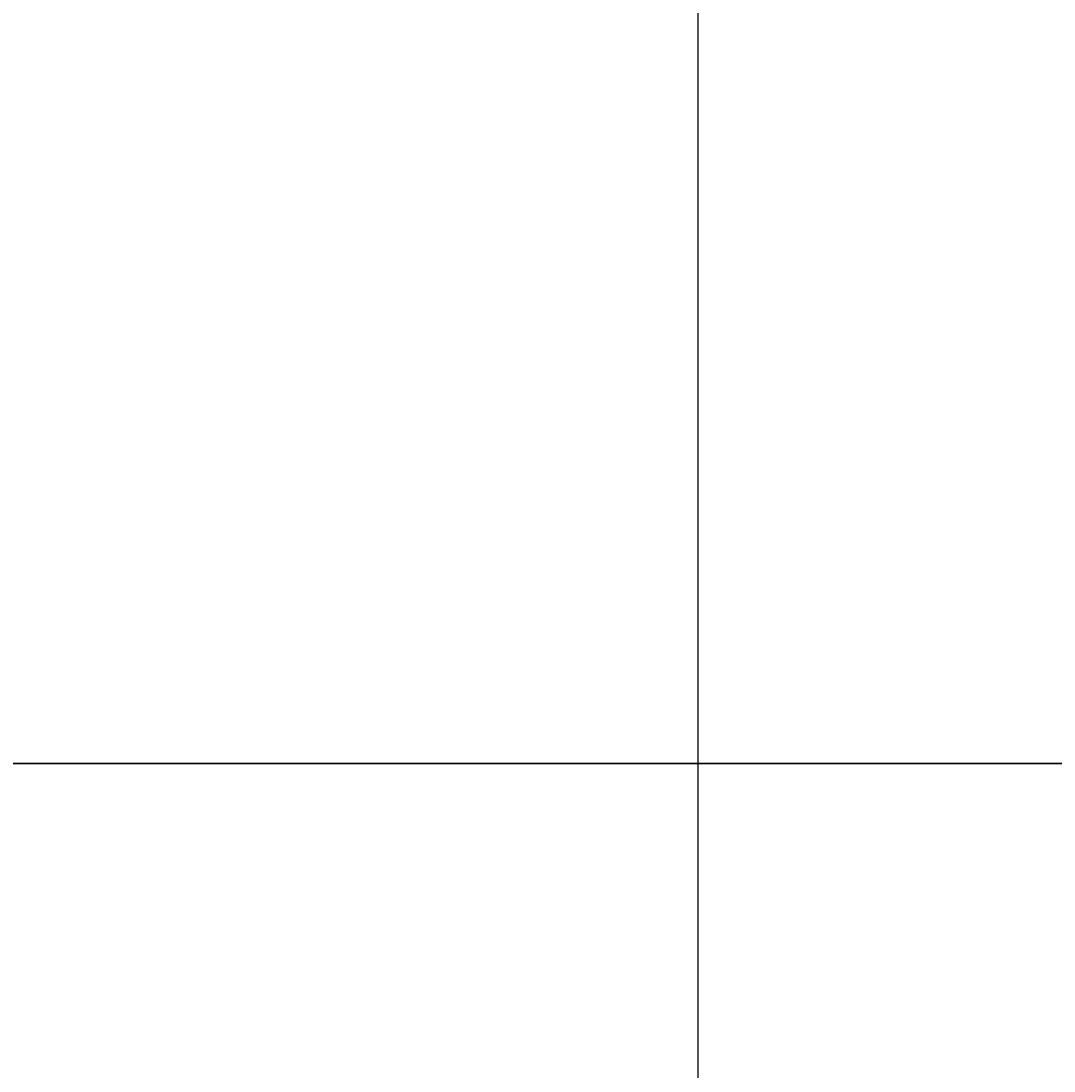
# Model space of a CAD drawing. Units: inches. Extents: x -6 to 289, y -8 to 323.
# Tile 84 of 107: x 173 to 196, y 252 to 276. Entities that reach past the tile are written whole.
import ezdxf

# ---------------------------------------------------------------- set-up
doc = ezdxf.new("R2010")
doc.units = ezdxf.units.IN
doc.header["$MEASUREMENT"] = 0
doc.layers.add('A-ANNO-DIMS', color=2, linetype='Continuous', lineweight=18)
doc.layers.add('A-ELEV', color=7, linetype='Continuous', lineweight=35)
doc.styles.get("Standard").update_dxf_attribs({"font": 'arial.ttf'})
doc.dimstyles.get("Standard").update_dxf_attribs({"dimtxt": 0.18, "dimasz": 0.18, "dimexe": 0.18, "dimexo": 0.0625, "dimgap": 0.09, "dimtad": 0, "dimtih": 1, "dimtoh": 1, "dimdec": 4, "dimzin": 0, "dimdsep": 46, "dimtxsty": 'Standard', "dimcen": 0.09, "dimadec": 0, "dimazin": 0, "dimtfac": 1, "dimtdec": 4, "dimtofl": 0, "dimtmove": 0, "dimatfit": 3, "dimfxl": 1, "dimtolj": 1, "dimtzin": 0, "dimarcsym": 0})

# ---------------------------------------------------------------- blocks, each defined once
blk = doc.blocks.new('*D12')
at = {"layer": 'A-ANNO-DIMS', "color": 0, "lineweight": -2, "transparency": 16777216}
for p, q in [((168.883, 226.717), (168.883, 322.969)), ((188.292, 226.951), (188.292, 322.969)), ((169.063, 322.789), (178.22, 322.789)), ((188.112, 322.789), (178.955, 322.789))]:
    blk.add_line(p, q, dxfattribs=at)
at = {"layer": 'A-ANNO-DIMS', "color": 0, "transparency": 16777216}
for points in [[(169.063, 322.819), (169.063, 322.759), (168.883, 322.789)], [(188.112, 322.819), (188.112, 322.759), (188.292, 322.789)]]:
    blk.add_solid(points, dxfattribs=at)
at = {"layer": 'Defpoints', "color": 0, "transparency": 16777216}
for p in [(188.292, 322.789), (188.292, 226.889), (168.883, 226.654)]:
    blk.add_point(p, dxfattribs=at)
at = {"layer": 'A-ANNO-DIMS', "color": 0, "transparency": 16777216, "insert": (178.588, 322.789), "char_height": 0.18, "attachment_point": 5}
blk.add_mtext('\\A1;19.41', dxfattribs=at)
blk = doc.blocks.new('*D13')
at = {"layer": 'A-ANNO-DIMS', "color": 0, "lineweight": -2, "transparency": 16777216}
for p, q in [((188.292, 226.951), (188.292, 322.969)), ((236.292, 226.951), (236.292, 322.969)), ((188.472, 322.789), (212.069, 322.789)), ((236.112, 322.789), (212.515, 322.789))]:
    blk.add_line(p, q, dxfattribs=at)
at = {"layer": 'A-ANNO-DIMS', "color": 0, "transparency": 16777216}
for points in [[(188.472, 322.819), (188.472, 322.759), (188.292, 322.789)], [(236.112, 322.819), (236.112, 322.759), (236.292, 322.789)]]:
    blk.add_solid(points, dxfattribs=at)
at = {"layer": 'Defpoints', "color": 0, "transparency": 16777216}
for p in [(236.292, 322.789), (188.292, 226.889), (236.292, 226.889)]:
    blk.add_point(p, dxfattribs=at)
at = {"layer": 'A-ANNO-DIMS', "color": 0, "transparency": 16777216, "insert": (212.292, 322.789), "char_height": 0.18, "attachment_point": 5}
blk.add_mtext('\\A1;48', dxfattribs=at)
blk = doc.blocks.new('*D27')
at = {"layer": 'A-ANNO-DIMS', "color": 0, "lineweight": -2, "transparency": 16777216}
for p, q in [((19.226, 307.289), (288.653, 307.289)), ((288.473, 307.109), (288.473, 277.471)), ((288.473, 247.469), (288.473, 277.107)), ((247.226, 247.289), (288.653, 247.289))]:
    blk.add_line(p, q, dxfattribs=at)
at = {"layer": 'A-ANNO-DIMS', "color": 0, "transparency": 16777216}
for points in [[(288.443, 307.109), (288.503, 307.109), (288.473, 307.289)], [(288.443, 247.469), (288.503, 247.469), (288.473, 247.289)]]:
    blk.add_solid(points, dxfattribs=at)
at = {"layer": 'Defpoints', "color": 0, "transparency": 16777216}
for p in [(19.164, 307.289), (288.473, 307.289), (247.164, 247.289)]:
    blk.add_point(p, dxfattribs=at)
at = {"layer": 'A-ANNO-DIMS', "color": 0, "transparency": 16777216, "insert": (288.473, 277.289), "char_height": 0.18, "attachment_point": 5}
blk.add_mtext('\\A1;60', dxfattribs=at)
blk = doc.blocks.new('*D79')
at = {"layer": 'A-ANNO-DIMS', "color": 0, "lineweight": -2, "transparency": 16777216}
for p, q in [((171.296, 118.033), (171.296, 322.969)), ((188.292, 116.842), (188.292, 322.969)), ((171.476, 322.789), (179.339, 322.789)), ((188.112, 322.789), (180.249, 322.789))]:
    blk.add_line(p, q, dxfattribs=at)
at = {"layer": 'A-ANNO-DIMS', "color": 0, "transparency": 16777216}
for points in [[(171.476, 322.819), (171.476, 322.759), (171.296, 322.789)], [(188.112, 322.819), (188.112, 322.759), (188.292, 322.789)]]:
    blk.add_solid(points, dxfattribs=at)
at = {"layer": 'Defpoints', "color": 0, "transparency": 16777216}
for p in [(188.292, 322.789), (171.296, 117.971), (188.292, 116.779)]:
    blk.add_point(p, dxfattribs=at)
at = {"layer": 'A-ANNO-DIMS', "color": 0, "transparency": 16777216, "insert": (179.794, 322.789), "char_height": 0.18, "attachment_point": 5}
blk.add_mtext('\\A1;16.996', dxfattribs=at)
blk = doc.blocks.new('*D80')
at = {"layer": 'A-ANNO-DIMS', "color": 0, "lineweight": -2, "transparency": 16777216}
for p, q in [((188.292, 116.842), (188.292, 322.969)), ((230.292, 116.842), (230.292, 322.969)), ((188.472, 322.789), (209.07, 322.789)), ((230.112, 322.789), (209.513, 322.789))]:
    blk.add_line(p, q, dxfattribs=at)
at = {"layer": 'A-ANNO-DIMS', "color": 0, "transparency": 16777216}
for points in [[(188.472, 322.819), (188.472, 322.759), (188.292, 322.789)], [(230.112, 322.819), (230.112, 322.759), (230.292, 322.789)]]:
    blk.add_solid(points, dxfattribs=at)
at = {"layer": 'Defpoints', "color": 0, "transparency": 16777216}
for p in [(230.292, 322.789), (188.292, 116.779), (230.292, 116.779)]:
    blk.add_point(p, dxfattribs=at)
at = {"layer": 'A-ANNO-DIMS', "color": 0, "transparency": 16777216, "insert": (209.292, 322.789), "char_height": 0.18, "attachment_point": 5}
blk.add_mtext('\\A1;42', dxfattribs=at)
blk = doc.blocks.new('*D96')
at = {"layer": 'A-ANNO-DIMS', "color": 0, "lineweight": -2, "transparency": 16777216}
for p, q in [((164.004, 159.411), (164.004, 322.969)), ((200.616, 159.411), (200.616, 322.969)), ((164.184, 322.789), (181.934, 322.789)), ((200.436, 322.789), (182.686, 322.789))]:
    blk.add_line(p, q, dxfattribs=at)
at = {"layer": 'A-ANNO-DIMS', "color": 0, "transparency": 16777216}
for points in [[(164.184, 322.819), (164.184, 322.759), (164.004, 322.789)], [(200.436, 322.819), (200.436, 322.759), (200.616, 322.789)]]:
    blk.add_solid(points, dxfattribs=at)
at = {"layer": 'Defpoints', "color": 0, "transparency": 16777216}
for p in [(200.616, 322.789), (164.004, 159.348), (200.616, 159.348)]:
    blk.add_point(p, dxfattribs=at)
at = {"layer": 'A-ANNO-DIMS', "color": 0, "transparency": 16777216, "insert": (182.31, 322.789), "char_height": 0.18, "attachment_point": 5}
blk.add_mtext('\\A1;36.61', dxfattribs=at)

msp = doc.modelspace()

# ---------------------------------------------------------------- linework, layer by layer
at = {"layer": 'A-ELEV'}
msp.add_line((115.1638, 259.2888), (271.1638, 259.2888), dxfattribs=at)

# ---------------------------------------------------------------- dimensions: what is measured, and where the dimension line sits
at = {"layer": 'A-ANNO-DIMS'}
for base, p1, p2, override, picture, middle in [((200.6162, 322.7888), (164.0039, 159.3484), (200.6162, 159.3484), {"dimdec": 2, "dimlfac": 1, "dimrnd": 0, "dimzin": 0, "dimdsep": 46, "dimlunit": 2}, '*D96', (182.3101, 322.7888)), ((188.2918, 322.7888), (168.8835, 226.654), (188.2918, 226.8887), {"dimdec": 2, "dimlfac": 1, "dimrnd": 0, "dimzin": 0, "dimdsep": 46, "dimlunit": 2}, '*D12', (178.5876, 322.7888)), ((188.2918, 322.7888), (171.296, 117.9706), (188.2918, 116.7795), {"dimdec": 3, "dimlfac": 1, "dimrnd": 0, "dimzin": 0, "dimdsep": 46, "dimlunit": 2}, '*D79', (179.7939, 322.7888)), ((236.2918, 322.7888), (188.2918, 226.8887), (236.2918, 226.8887), {"dimdec": 0, "dimlfac": 1, "dimrnd": 0, "dimzin": 0, "dimdsep": 46, "dimlunit": 2}, '*D13', (212.2918, 322.7888)), ((230.2918, 322.7888), (188.2918, 116.7795), (230.2918, 116.7795), {"dimdec": 0, "dimlfac": 1, "dimrnd": 0, "dimzin": 0, "dimdsep": 46, "dimlunit": 2}, '*D80', (209.2918, 322.7888))]:
    dim = msp.add_linear_dim(base=base, p1=p1, p2=p2, dimstyle='Standard', override=override, dxfattribs=at)
    dim.commit()
    dim.dimension.update_dxf_attribs({"geometry": picture, "text_midpoint": middle})
dim = msp.add_linear_dim(base=(288.4733, 307.2888), p1=(247.1638, 247.2888), p2=(19.1638, 307.2888), angle=90, dimstyle='Standard', override={"dimdec": 0, "dimlfac": 1, "dimrnd": 0, "dimzin": 0, "dimdsep": 46, "dimlunit": 2}, dxfattribs=at)
dim.commit()
dim.dimension.update_dxf_attribs({"geometry": '*D27', "text_midpoint": (288.4733, 277.2888)})

doc.saveas('drawing.dxf')
